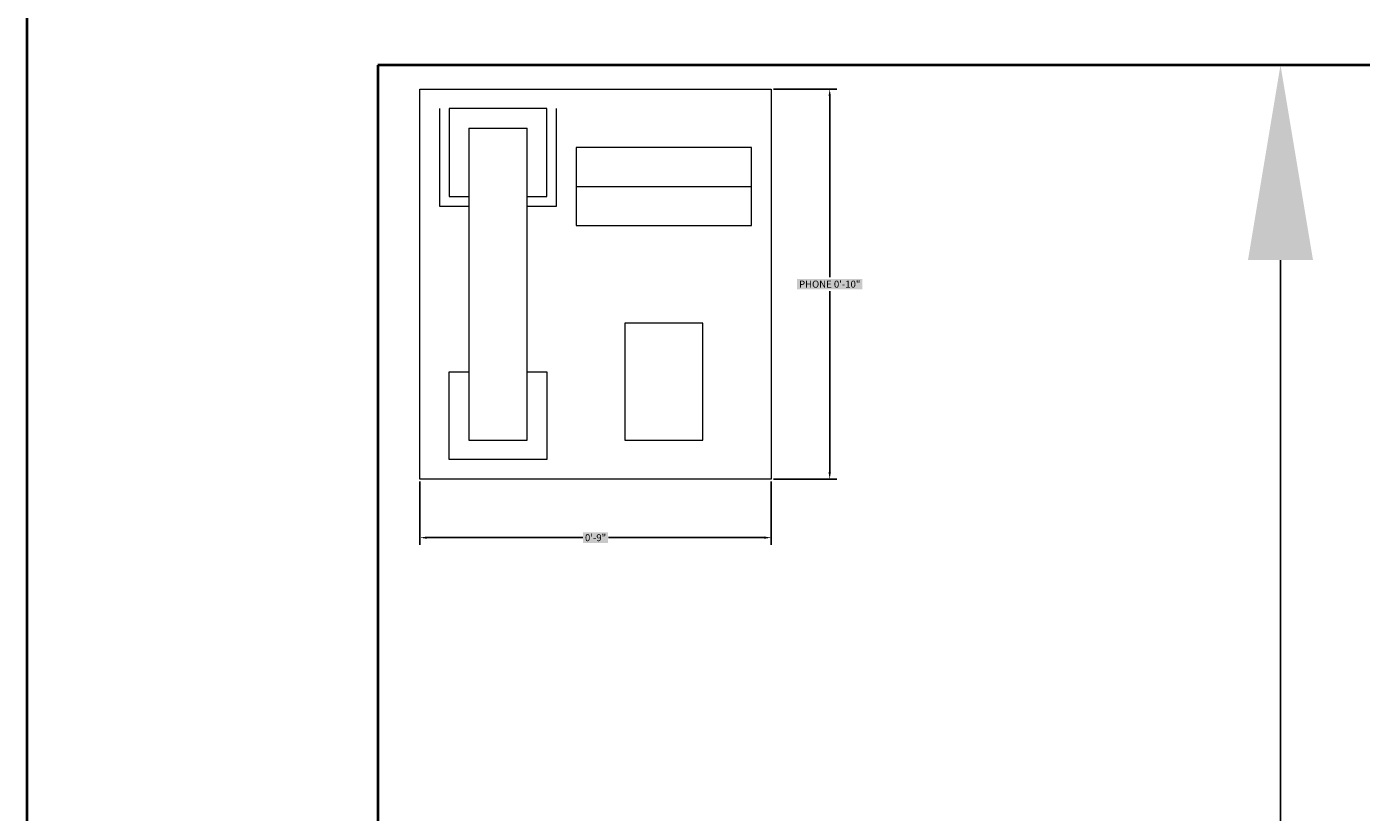
# Model space of a CAD drawing. Units: inches. Extents: x -301 to 715, y -607 to 364.
# Tile 75 of 141: x -205 to -170, y 47 to 67. Entities that reach past the tile are written whole.
import ezdxf

# ---------------------------------------------------------------- set-up
doc = ezdxf.new("R2010")
doc.units = ezdxf.units.IN
doc.header["$MEASUREMENT"] = 0
for name, color, linetype, lineweight in [('A-ANNO-DIMS', 2, 'Continuous', 18), ('A-FURN', 8, 'Continuous', 18), ('A-WALL', 3, 'Continuous', 40)]:
    doc.layers.add(name, color=color, linetype=linetype, lineweight=lineweight)
doc.styles.get("Standard").update_dxf_attribs({"font": 'arial.ttf'})
doc.dimstyles.get("Standard").update_dxf_attribs({"dimtxt": 0.18, "dimasz": 0.18, "dimexe": 0.18, "dimexo": 0.0625, "dimgap": 0.09, "dimtad": 0, "dimtih": 1, "dimtoh": 1, "dimdec": 1, "dimzin": 0, "dimdsep": 46, "dimlunit": 4, "dimtxsty": 'Standard', "dimcen": 0.09, "dimclrd": 3, "dimclre": 4, "dimclrt": 6, "dimadec": 0, "dimazin": 0, "dimtfac": 1, "dimtdec": 1, "dimtofl": 0, "dimtmove": 0, "dimatfit": 3, "dimfxl": 1, "dimtfill": 2, "dimtfillclr": 51, "dimtolj": 1, "dimtzin": 0, "dimarcsym": 0})

# ---------------------------------------------------------------- blocks, each defined once
blk = doc.blocks.new('Phone - Desk')
for p, q in [((-4.5, -5), (-4.5, 5)), ((-4.5, 5), (4.5, 5)), ((4.5, 5), (4.5, -5)), ((-4, 4.5), (-4, 2)), ((-3.75, 4.5), (-3.75, 2.25)), ((-1.25, 4.5), (-3.75, 4.5)), ((-1.25, 2.25), (-1.25, 4.5)), ((-1, 2), (-1, 4.5)), ((-3.25, 4), (-3.25, -4)), ((-3.25, 4), (-1.75, 4)), ((-1.75, -4), (-1.75, 4)), ((4, 3.5), (-0.5, 3.5)), ((-0.5, 3.5), (-0.5, 1.5)), ((4, 1.5), (4, 3.5)), ((-0.5, 2.5), (4, 2.5)), ((-3.75, 2.25), (-3.25, 2.25)), ((-1.75, 2.25), (-1.25, 2.25)), ((-4, 2), (-3.25, 2)), ((-1.75, 2), (-1, 2)), ((-0.5, 1.5), (4, 1.5)), ((2.75, -1), (0.75, -1)), ((0.75, -1), (0.75, -4)), ((2.75, -4), (2.75, -1)), ((-3.75, -2.25), (-3.25, -2.25)), ((-3.75, -4.5), (-3.75, -2.25)), ((-1.75, -2.25), (-1.25, -2.25)), ((-1.25, -2.25), (-1.25, -4.5)), ((-3.25, -4), (-1.75, -4)), ((0.75, -4), (2.75, -4)), ((-1.25, -4.5), (-3.75, -4.5)), ((4.5, -5), (-4.5, -5))]:
    blk.add_line(p, q)
blk = doc.blocks.new('*D56')
at = {"layer": 'A-ANNO-DIMS', "color": 0, "lineweight": -2, "transparency": 16777216}
for p, q in [((-195.541, 65.682), (-172.295, 65.682)), ((-172.475, 60.682), (-172.475, 0.778)), ((-172.475, -62.318), (-172.475, -2.414)), ((-195.541, -67.318), (-172.295, -67.318))]:
    blk.add_line(p, q, dxfattribs=at)
at = {"layer": 'A-ANNO-DIMS', "color": 0, "transparency": 16777216}
for points in [[(-173.308, 60.682), (-171.641, 60.682), (-172.475, 65.682)], [(-173.308, -62.318), (-171.641, -62.318), (-172.475, -67.318)]]:
    blk.add_solid(points, dxfattribs=at)
at = {"layer": 'Defpoints', "color": 0, "transparency": 16777216}
for p in [(-195.603, 65.682), (-172.475, 65.682), (-195.603, -67.318)]:
    blk.add_point(p, dxfattribs=at)
at = {"layer": 'A-ANNO-DIMS', "color": 0, "transparency": 16777216, "insert": (-172.475, -0.818), "char_height": 3, "attachment_point": 5, "bg_fill": 1, "box_fill_scale": 1.25, "bg_fill_color": 51, "bg_fill_transparency": 0}
blk.add_mtext('\\A1;11\'-1"', dxfattribs=at)
blk = doc.blocks.new('*D138')
at = {"layer": 'A-ANNO-DIMS', "color": 4, "lineweight": -2, "transparency": 16777216}
for p, q in [((-185.463, 65.065), (-183.846, 65.065)), ((-185.463, 55.065), (-183.846, 55.065))]:
    blk.add_line(p, q, dxfattribs=at)
at = {"layer": 'A-ANNO-DIMS', "color": 3, "lineweight": -2, "transparency": 16777216}
for p, q in [((-184.026, 64.885), (-184.026, 60.248)), ((-184.026, 55.245), (-184.026, 59.882))]:
    blk.add_line(p, q, dxfattribs=at)
at = {"layer": 'A-ANNO-DIMS', "color": 3, "transparency": 16777216}
for points in [[(-184.056, 64.885), (-183.996, 64.885), (-184.026, 65.065)], [(-184.056, 55.245), (-183.996, 55.245), (-184.026, 55.065)]]:
    blk.add_solid(points, dxfattribs=at)
at = {"layer": 'Defpoints', "color": 0, "transparency": 16777216}
for p in [(-185.526, 65.065), (-184.026, 65.065), (-185.526, 55.065)]:
    blk.add_point(p, dxfattribs=at)
at = {"layer": 'A-ANNO-DIMS', "color": 6, "transparency": 16777216, "insert": (-184.026, 60.065), "char_height": 0.18, "attachment_point": 5, "bg_fill": 1, "box_fill_scale": 1.25, "bg_fill_color": 51, "bg_fill_transparency": 0}
blk.add_mtext('\\A1;PHONE 0\'-10"', dxfattribs=at)
blk = doc.blocks.new('*D139')
at = {"layer": 'A-ANNO-DIMS', "color": 4, "lineweight": -2, "transparency": 16777216}
for p, q in [((-194.526, 55.003), (-194.526, 53.385)), ((-185.526, 55.003), (-185.526, 53.385))]:
    blk.add_line(p, q, dxfattribs=at)
at = {"layer": 'A-ANNO-DIMS', "color": 3, "lineweight": -2, "transparency": 16777216}
for p, q in [((-194.346, 53.565), (-190.355, 53.565)), ((-185.706, 53.565), (-189.696, 53.565))]:
    blk.add_line(p, q, dxfattribs=at)
at = {"layer": 'A-ANNO-DIMS', "color": 3, "transparency": 16777216}
for points in [[(-194.346, 53.595), (-194.346, 53.535), (-194.526, 53.565)], [(-185.706, 53.595), (-185.706, 53.535), (-185.526, 53.565)]]:
    blk.add_solid(points, dxfattribs=at)
at = {"layer": 'Defpoints', "color": 0, "transparency": 16777216}
for p in [(-194.526, 55.065), (-185.526, 55.065), (-185.526, 53.565)]:
    blk.add_point(p, dxfattribs=at)
at = {"layer": 'A-ANNO-DIMS', "color": 6, "transparency": 16777216, "insert": (-190.026, 53.565), "char_height": 0.18, "attachment_point": 5, "bg_fill": 1, "box_fill_scale": 1.25, "bg_fill_color": 51, "bg_fill_transparency": 0}
blk.add_mtext('\\A1;0\'-9"', dxfattribs=at)
blk = doc.blocks.new('*D151')
at = {"layer": 'A-ANNO-DIMS', "color": 4, "lineweight": -2, "transparency": 16777216}
for p, q in [((-204.603, -223.755), (-204.603, 359.612)), ((-45.603, -214.755), (-45.603, 359.612))]:
    blk.add_line(p, q, dxfattribs=at)
at = {"layer": 'A-ANNO-DIMS', "color": 3, "lineweight": -2, "transparency": 16777216}
for p, q in [((-204.423, 359.432), (-125.494, 359.432)), ((-45.783, 359.432), (-124.713, 359.432))]:
    blk.add_line(p, q, dxfattribs=at)
at = {"layer": 'A-ANNO-DIMS', "color": 3, "transparency": 16777216}
for points in [[(-204.423, 359.462), (-204.423, 359.402), (-204.603, 359.432)], [(-45.783, 359.462), (-45.783, 359.402), (-45.603, 359.432)]]:
    blk.add_solid(points, dxfattribs=at)
at = {"layer": 'Defpoints', "color": 0, "transparency": 16777216}
for p in [(-45.603, 359.432), (-45.603, -214.818), (-204.603, -223.818)]:
    blk.add_point(p, dxfattribs=at)
at = {"layer": 'A-ANNO-DIMS', "color": 6, "transparency": 16777216, "insert": (-125.103, 359.432), "char_height": 0.18, "attachment_point": 5, "bg_fill": 1, "box_fill_scale": 1.25, "bg_fill_color": 51, "bg_fill_transparency": 0}
blk.add_mtext('\\A1;13\'-3"', dxfattribs=at)

msp = doc.modelspace()

# ---------------------------------------------------------------- linework, layer by layer
at = {"layer": 'A-WALL'}
for p, q in [((-204.603, 71.682), (-204.603, -67.318)), ((-45.603, 65.682), (-195.603, 65.682)), ((-195.603, 65.682), (-195.603, -67.318))]:
    msp.add_line(p, q, dxfattribs=at)

# ---------------------------------------------------------------- block references
at = {"layer": 'A-FURN'}
msp.add_blockref('Phone - Desk', (-190.026, 60.065), dxfattribs=at)

# ---------------------------------------------------------------- dimensions: what is measured, and where the dimension line sits
at = {"layer": 'A-ANNO-DIMS'}
for base, p1, p2, picture, middle in [((-45.603, 359.432), (-204.603, -223.818), (-45.603, -214.818), '*D151', (-125.103, 359.432)), ((-185.526, 53.565), (-194.526, 55.065), (-185.526, 55.065), '*D139', (-190.026, 53.565))]:
    dim = msp.add_linear_dim(base=base, p1=p1, p2=p2, dimstyle='Standard', override={"dimdec": 1, "dimlfac": 1, "dimrnd": 0, "dimzin": 1, "dimdsep": 46, "dimlunit": 4, "dimfrac": 2}, dxfattribs=at)
    dim.commit()
    dim.dimension.update_dxf_attribs({"geometry": picture, "text_midpoint": middle})
dim = msp.add_linear_dim(base=(-172.475, 65.682), p1=(-195.603, -67.318), p2=(-195.603, 65.682), angle=90, dimstyle='Standard', override={"dimtxt": 3, "dimasz": 5, "dimclrd": 0, "dimclre": 0, "dimclrt": 0}, dxfattribs=at)
dim.commit()
dim.dimension.update_dxf_attribs({"geometry": '*D56', "text_midpoint": (-172.475, -0.818)})
dim = msp.add_linear_dim(base=(-184.026, 65.065), p1=(-185.526, 55.065), p2=(-185.526, 65.065), angle=90, text='PHONE <>', dimstyle='Standard', override={"dimdec": 1, "dimlfac": 1, "dimrnd": 0, "dimzin": 1, "dimdsep": 46, "dimlunit": 4, "dimfrac": 2}, dxfattribs=at)
dim.commit()
dim.dimension.update_dxf_attribs({"geometry": '*D138', "text_midpoint": (-184.026, 60.065)})

doc.saveas('drawing.dxf')
